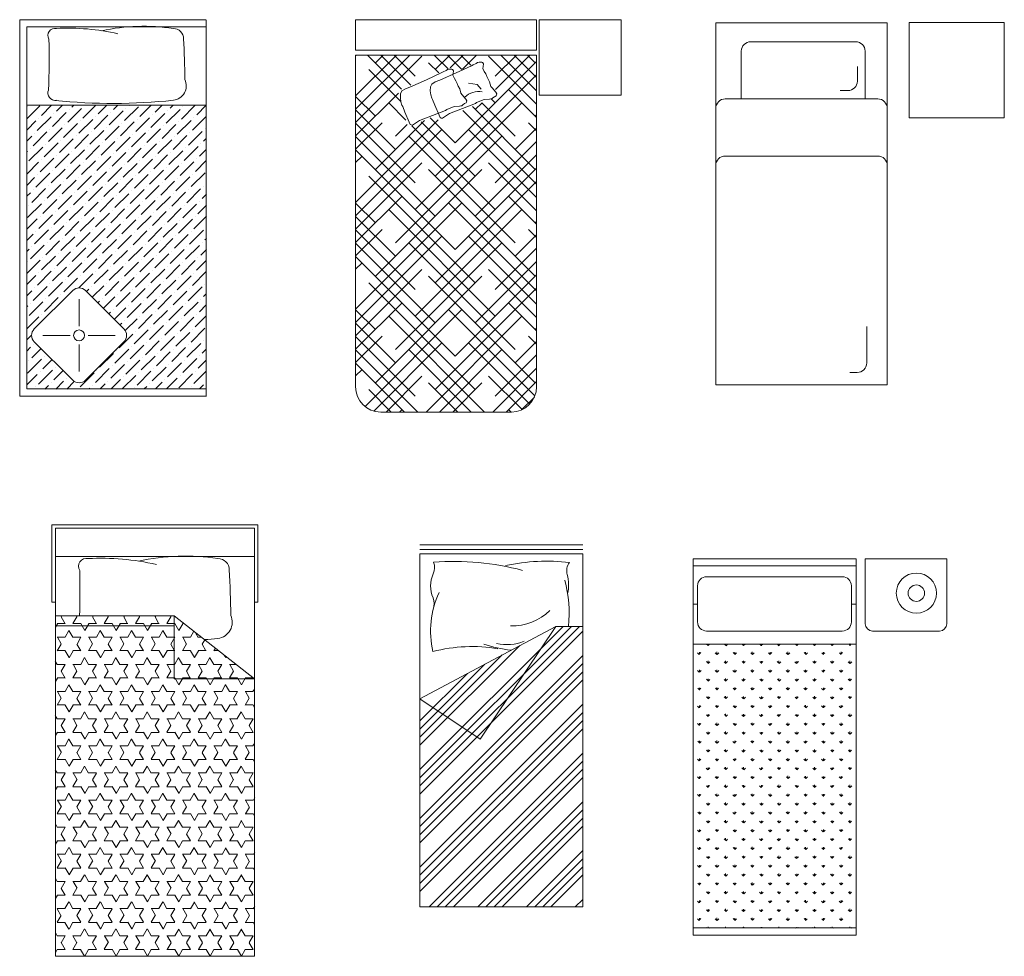
# Model space of a CAD drawing. Units: inches. Extents: x 1994 to 3075, y 3517 to 3950.
# Tile 20 of 58: x 1994.5453 to 1994.7595, y 3553.3484 to 3553.5521. Entities that reach past the tile are written whole.
import ezdxf

# ---------------------------------------------------------------- set-up
doc = ezdxf.new("R2010")
doc.units = ezdxf.units.IN
doc.layers.add('A-FURN-REFR', color=8, linetype='Continuous', lineweight=13)
doc.layers.add('A-FURN-REFR-PATT', color=8, linetype='Continuous', lineweight=13)

# ---------------------------------------------------------------- blocks, each defined once
blk = doc.blocks.new('*X5')
at = {"color": 0}
for p, q in [((-210.7580465308878, 409.7281539603075), (-199.9708546801334, 420.5153458110619)), ((-210.7580465308878, 412.379804389757), (-202.6225051095829, 420.5153458110619)), ((-210.7580465308878, 420.3347556781058), (-210.5774563979316, 420.5153458110619)), ((-210.7580465308878, 407.076503530858), (-197.547956993992, 420.2865930677537)), ((-201.617062875051, 413.7490972310152), (-208.3833114550977, 420.5153458110619)), ((-206.8287334970653, 418.9607678530292), (-205.2741555390325, 420.5153458110619)), ((-199.7682837993056, 414.5519685847194), (-205.7316610256482, 420.5153458110619)), ((-198.8737822087164, 416.3091174235798), (-203.0800105961986, 420.515345811062)), ((-192.3731674963244, 417.7634539995364), (-195.12505930785, 420.5153458110619)), ((-194.8963065645422, 417.6349426383045), (-192.0159033917846, 420.515345811062)), ((-189.6311998323742, 417.6731367650358), (-192.4734088784004, 420.515345811062)), ((-191.9188461243063, 417.9607526490907), (-189.3642529623351, 420.5153458110619)), ((-190.9188309203679, 403.0508652763318), (-174.7580465308877, 419.211649665812)), ((-187.8124935512899, 418.5060809134011), (-189.8217584489508, 420.5153458110619)), ((-189.4902654306947, 417.7376829132529), (-186.7126025328856, 420.5153458110619)), ((-174.7580465308877, 410.7549347518979), (-184.2897048467439, 420.2865930677541)), ((-182.9638796320193, 416.3091174235796), (-178.7576512445369, 420.5153458110619)), ((-182.9257945198644, 413.695552106285), (-176.1060008150873, 420.515345811062)), ((-174.7580465308877, 413.4065851813475), (-181.8668071606022, 420.5153458110619)), ((-174.7580465308877, 416.058235610797), (-179.2151567311527, 420.5153458110619)), ((-175.0089283436705, 418.9607678530292), (-176.5635063017031, 420.5153458110619)), ((-201.7778662022018, 411.2582501287165), (-208.1545587117899, 417.6349426383045)), ((-194.2219465720697, 416.9605826458322), (-196.2221317792669, 418.9607678530292)), ((-194.8963065645423, 396.421739202708), (-174.7580465308877, 416.5599992363624)), ((-174.7580465308877, 408.1032843224484), (-180.3122292025696, 413.6574669941301)), ((-210.7580465308878, 404.4248531014084), (-202.2434538897721, 412.9394457425241)), ((-206.8287334970651, 408.3541661352311), (-210.7580465308878, 412.2834791690537)), ((-182.9638796320191, 411.0058165646806), (-183.727333396784, 411.7692703294456)), ((-202.8512578528907, 401.7250400616072), (-210.7580465308877, 409.6318287396042)), ((-200.7622625975809, 407.590996094646), (-204.1770830676156, 411.0058165646806)), ((-198.8737822087168, 389.7926131290839), (-177.6605787731203, 411.0058165646803)), ((-174.7580465308877, 394.8450321752006), (-189.4137563576908, 409.5007420020037)), ((-175.0089283436705, 397.7475644174329), (-187.5182820373886, 410.256918111151)), ((-186.9413552761936, 409.6799913499556), (-185.5985917406192, 411.02275488553)), ((-178.9864039878448, 404.3766904910567), (-185.6228077170863, 411.0130942202982)), ((-210.7580465308878, 391.1666009541607), (-194.3064165629733, 407.6182309220751)), ((-206.8287334970653, 397.7475644174327), (-197.0508686209985, 407.5254292934994)), ((-190.9188309203678, 403.050865276332), (-195.8995790361304, 408.0316133920946)), ((-175.0089283436706, 408.3541661352309), (-174.7580465308877, 408.6050479480137)), ((-210.7580465308878, 401.7732026719589), (-205.5029082823405, 407.0283409205061)), ((-198.8737822087164, 395.0959139879834), (-210.7580465308878, 406.9801783101546)), ((-210.7580465308878, 388.5149505247111), (-193.5704813498175, 405.7025157057813)), ((-202.851257852891, 404.3766904910565), (-200.5182087880894, 406.7097395558581)), ((-182.9638796320191, 389.7926131290843), (-199.583278575489, 406.4120120725541)), ((-186.9413552761934, 396.4217392027081), (-197.7414288058097, 407.2218127323244)), ((-174.7580465308877, 392.1933817457511), (-188.2671804909182, 405.7025157057815)), ((-178.9864039878449, 401.7250400616069), (-174.7580465308877, 405.9533975185642)), ((-174.7580465308877, 405.4516338929988), (-176.3347535583952, 407.0283409205063)), ((-194.8963065645421, 388.4667879143594), (-210.7580465308878, 404.328527880705)), ((-202.8512578528911, 383.16348705546), (-181.6380544172947, 404.3766904910564)), ((-178.9864039878448, 383.1634870554603), (-200.1996074234412, 404.3766904910567)), ((-190.9188309203678, 381.8376618407356), (-210.7580465308878, 401.6768774512555)), ((-182.9638796320193, 395.0959139879831), (-174.7580465308877, 403.3017470891146)), ((-210.7580465308878, 399.1215522425094), (-209.4803839265148, 400.3992148468823)), ((-186.9413552761938, 388.4667879143591), (-174.7580465308877, 400.6500966596651)), ((-210.7580465308878, 385.8633000952616), (-197.5479569939918, 399.0733896321575)), ((-206.8287334970653, 376.5343609818363), (-185.6155300614688, 397.7475644174327)), ((-175.0089283436705, 376.5343609818365), (-196.2221317792669, 397.7475644174329)), ((-190.9188309203679, 381.8376618407354), (-174.7580465308877, 397.9984462302155)), ((-174.7580465308877, 389.5417313163016), (-184.2897048467439, 399.0733896321577)), ((-186.9413552761934, 375.2085357671117), (-208.1545587117898, 396.4217392027081)), ((-194.8963065645423, 375.2085357671115), (-174.7580465308877, 395.346795800766)), ((-210.7580465308878, 383.211649665812), (-201.5254326381662, 392.4442635585336)), ((-174.7580465308877, 386.890080886852), (-180.3122292025696, 392.4442635585338)), ((-210.7580465308878, 369.9533975185643), (-189.5930057056432, 391.1184383438088)), ((-206.8287334970651, 387.1409626996347), (-210.7580465308878, 391.0702757334573)), ((-182.9638796320191, 368.5794096934878), (-204.1770830676156, 389.7926131290843)), ((-198.8737822087166, 368.5794096934876), (-177.6605787731202, 389.792613129084)), ((-174.7580465308877, 373.6318287396042), (-192.2446561350925, 391.118438343809)), ((-202.8512578528907, 380.5118366260108), (-210.7580465308877, 388.4186253040078)), ((-175.0089283436706, 387.1409626996345), (-174.7580465308877, 387.3918445124174)), ((-210.7580465308878, 380.5599992363625), (-205.5029082823405, 385.8151374849098)), ((-198.8737822087164, 373.8827105523869), (-210.7580465308877, 385.7669748745582)), ((-210.7580465308878, 367.3017470891147), (-193.5704813498175, 384.4893122701849)), ((-174.7580465308877, 370.9801783101547), (-188.2671804909182, 384.4893122701852)), ((-178.986403987845, 380.5118366260106), (-174.7580465308878, 384.7401940829678)), ((-174.7580465308877, 384.2384304574025), (-176.3347535583952, 385.81513748491)), ((-194.8963065645421, 367.253584478763), (-210.7580465308878, 383.1153244451087)), ((-202.8512578528909, 361.9502836198638), (-181.6380544172945, 383.1634870554602)), ((-178.9864039878448, 361.9502836198639), (-200.1996074234412, 383.1634870554603)), ((-182.9638796320192, 373.8827105523869), (-174.7580465308877, 382.0885436535184)), ((-190.9188309203678, 360.6244584051392), (-210.7580465308877, 380.4636740156592)), ((-210.7580465308878, 377.9083488069129), (-209.480383926515, 379.1860114112858)), ((-186.9413552761936, 367.2535844787628), (-174.7580465308877, 379.4368932240687)), ((-210.7580465308878, 364.6500966596652), (-197.547956993992, 377.8601861965609)), ((-206.8287334970653, 355.3211575462399), (-185.6155300614688, 376.5343609818363)), ((-175.0089283436705, 355.32115754624), (-196.2221317792669, 376.5343609818365)), ((-190.9188309203679, 360.624458405139), (-174.7580465308877, 376.7852427946191)), ((-174.7580465308877, 368.3285278807051), (-184.2897048467439, 377.8601861965612)), ((-186.9413552761935, 353.9953323315153), (-208.1545587117899, 375.2085357671118)), ((-194.8963065645423, 353.9953323315151), (-174.7580465308878, 374.1335923651696)), ((-210.7580465308878, 361.9984462302156), (-201.5254326381662, 371.2310601229372)), ((-174.7580465308877, 365.6768774512556), (-180.3122292025696, 371.2310601229374)), ((-206.8287334970651, 365.9277592640383), (-210.7580465308877, 369.8570722978609)), ((-208.8846967480148, 350.6135438658409), (-189.5930057056432, 369.9052349082124)), ((-185.1130191851898, 349.5153458110621), (-204.1770830676156, 368.5794096934878)), ((-196.7246426555458, 349.5153458110621), (-177.6605787731202, 368.5794096934877)), ((-175.0826291794211, 352.7432079525412), (-192.2446561350925, 369.9052349082126)), ((-202.8512578528908, 359.2986331904144), (-210.7580465308877, 367.2054218684114)), ((-210.7580465308878, 359.3467958007661), (-205.5029082823405, 364.6019340493134)), ((-198.8737822087165, 352.6695071167905), (-210.7580465308878, 364.5537714389618)), ((-174.7580465308877, 363.025227021806), (-176.3347535583952, 364.6019340493135)), ((-175.0089283436707, 365.9277592640381), (-174.7580465308878, 366.1786410768209)), ((-207.1372587068342, 349.7093314775719), (-193.5704813498174, 363.2761088345887)), ((-176.0989374029306, 351.1078657466011), (-188.2671804909182, 363.2761088345887)), ((-178.986403987845, 359.2986331904143), (-174.7580465308878, 363.5269906473715)), ((-198.3712713324375, 349.5153458110621), (-210.7580465308878, 361.9021210095123)), ((-187.7646696146393, 349.5153458110621), (-200.1996074234413, 361.950283619864)), ((-194.0729922260963, 349.5153458110621), (-181.6380544172946, 361.9502836198638)), ((-182.9638796320193, 352.6695071167903), (-174.7580465308878, 360.8753402179218)), ((-201.0229217618871, 349.5153458110621), (-210.7580465308878, 359.2504705800627)), ((-210.7580465308878, 356.6951453713165), (-209.4803839265148, 357.9728079756894)), ((-204.6795939438944, 349.5153458110621), (-197.5479569939918, 356.6469827609647)), ((-177.6324032389686, 349.9896811531895), (-184.2897048467439, 356.6469827609648)), ((-183.4663905082981, 349.5153458110621), (-174.7580465308878, 358.2236897884723)), ((-190.4163200440889, 349.5153458110621), (-196.2221317792669, 355.3211575462401)), ((-191.4213417966468, 349.5153458110621), (-185.6155300614689, 355.3211575462399)), ((-180.8147400788485, 349.5153458110621), (-174.7580465308878, 355.5720393590228)), ((-203.6745721913366, 349.5153458110621), (-208.1545587117899, 353.9953323315153)), ((-177.7359644727731, 349.942470987688), (-175.1851717075138, 352.4932637529473)), ((-202.0279435144449, 349.5153458110621), (-201.5254326381662, 350.0178566873408)), ((-179.8097183262906, 349.5153458110621), (-180.3122292025696, 350.017856687341))]:
    blk.add_line(p, q, dxfattribs=at)

msp = doc.modelspace()

# ---------------------------------------------------------------- hatches: boundary and pattern name
at = {"layer": 'A-FURN-REFR-PATT'}
h = msp.add_hatch(dxfattribs=at)
h.set_pattern_fill('ANSI36', color=256, scale=0.0005368647100931, style=0)
h.set_pattern_definition([(45, (1992.896359554233, 3553.126432773951), (0.0009039717373123, 0.0033145630368119), [0.0042613636363636, -0.0008522727272727, 0, -0.0008522727272727])])
h.paths.add_polyline_path([(1994.546861451254, 3553.471827593295), (1994.585872349944, 3553.471827593295), (1994.585872349944, 3553.533572260688), (1994.546861451254, 3553.533572260688)])
h.paths.add_polyline_path([(1994.559597014725, 3553.493218537151), (1994.567948669621, 3553.484866882255, -0.4142135623730951), (1994.567948669621, 3553.48208299729), (1994.559597014725, 3553.473731342394, -0.4142135623730951), (1994.55681312976, 3553.473731342394), (1994.548461474864, 3553.48208299729, -0.4142135623730951), (1994.548461474864, 3553.484866882255), (1994.55681312976, 3553.493218537151, -0.4142135623730949)], flags=16)
h = msp.add_hatch(dxfattribs=at)
h.set_pattern_fill('STARS', color=256, scale=0.0005368647100931, style=0)
h.set_pattern_definition([(0, (1993.050049029089, 3553.090100364233), (0, 0.0029523586256263), [0.0017045454545455, -0.0017045454545455]), (60, (1993.050049029089, 3553.090100364233), (-0.0025568175708745, 0.0014761793128132), [0.0017045454545455, -0.0017045454545455]), (119.9999999999999, (1993.050901301817, 3553.091576543546), (-0.0025568175708745, -0.0014761793128132), [0.0017045454545455, -0.0017045454545455])])
h.paths.add_polyline_path([(1994.553043561207, 3553.348413258822), (1994.596372491915, 3553.348413258822), (1994.596372491915, 3553.408773288821), (1994.578910061208, 3553.408773288821), (1994.578910061208, 3553.420293288821), (1994.553043561207, 3553.420293288821)])
h.paths.add_polyline_path([(1994.596372491915, 3553.408773288821), (1994.578910061208, 3553.422453288821), (1994.578910061208, 3553.408773288821)])
h.paths.add_polyline_path([(1994.578910061208, 3553.420293288821), (1994.578910061208, 3553.422453288821), (1994.553043561207, 3553.422453288821), (1994.553043561207, 3553.420293288821)])
h = msp.add_hatch(dxfattribs=at)
h.set_pattern_fill('ANSI34', color=256, scale=0.0003937007874016, style=0)
h.set_pattern_definition([(45, (1993.050049029089, 3553.090100364233), (-0.0053033008588991, 0.0053033008588991), []), (45, (1993.051816796806, 3553.090100364233), (-0.0053033008588991, 0.0053033008588991), []), (45, (1993.053584564523, 3553.090100364233), (-0.0053033008588991, 0.0053033008588991), []), (45, (1993.055352336176, 3553.090100364233), (-0.0053033008588991, 0.0053033008588991), [])])
h.paths.add_polyline_path([(1994.632359589973, 3553.404436820766), (1994.645437540004, 3553.395663695953), (1994.661887149027, 3553.420184852262)], flags=17)
h.paths.add_polyline_path([(1994.645437540004, 3553.395663695953), (1994.632359589973, 3553.404436820766), (1994.632359589973, 3553.359161230215), (1994.667792660839, 3553.359161230215), (1994.667792660839, 3553.420184852262), (1994.661887149027, 3553.420184852262)])
h = msp.add_hatch(dxfattribs=at)
h.set_pattern_fill('GRASS', color=256, scale=0.0001073729420186, style=0)
h.set_pattern_definition([(90, (1993.050049029089, 3553.090100364233), (-0.0019284717251253, 0.0019284717251253), [0.0005113636363636, -0.0033455798138869]), (45, (1993.050049029089, 3553.090100364233), (-0.0019284730395997, 0.0019284730395997), [0.0005113636363636, -0.0022159090909091]), (135, (1993.050049029089, 3553.090100364233), (-0.0019284730395997, -0.0019284730395997), [0.0005113636363636, -0.0022159090909091])])
h.paths.add_polyline_path([(1994.69181488028, 3553.354574789245), (1994.727247951146, 3553.354574789245), (1994.727247951146, 3553.416319456637), (1994.69181488028, 3553.416319456637)])

# ---------------------------------------------------------------- linework, layer by layer
at = {"layer": 'A-FURN-REFR'}
for p, q in [((1994.545286648104, 3553.470252790145), (1994.545286648104, 3553.552142553924)), ((1994.585872349944, 3553.552142553924), (1994.545286648104, 3553.552142553924)), ((1994.546861451254, 3553.471827593295), (1994.546861451254, 3553.550567750775)), ((1994.585872349944, 3553.550567750775), (1994.546861451254, 3553.550567750775)), ((1994.585872349944, 3553.470157443203), (1994.585872349944, 3553.552047206982)), ((1994.696695721813, 3553.551494491247), (1994.733993691145, 3553.551494491247)), ((1994.696695721813, 3553.472754333767), (1994.696695721813, 3553.551494491247)), ((1994.733993691145, 3553.472754333767), (1994.733993691145, 3553.551494491247)), ((1994.696695721813, 3553.536989725396), (1994.696695721813, 3553.54942238184)), ((1994.727127375017, 3553.547351280916), (1994.704334171536, 3553.547351280916)), ((1994.702262062128, 3553.534918624472), (1994.702262062128, 3553.545279171509)), ((1994.729199484424, 3553.534918624472), (1994.729199484424, 3553.545279171509)), ((1994.727496280641, 3553.541967400785), (1994.727496280641, 3553.538785783707)), ((1994.642927317379, 3553.538302041658), (1994.64481344291, 3553.538032798672)), ((1994.64481344291, 3553.538032798672), (1994.645655457301, 3553.537023135932)), ((1994.723796114248, 3553.536713674299), (1994.725424171233, 3553.536713674299)), ((1994.585872349944, 3553.533572260688), (1994.546861451254, 3553.533572260688)), ((1994.69876783122, 3553.534917615988), (1994.731921581738, 3553.534917615988)), ((1994.69876783122, 3553.522484959544), (1994.731921581738, 3553.522484959544)), ((1994.55681312976, 3553.493218537151), (1994.548461474864, 3553.484866882255)), ((1994.567948669621, 3553.484866882255), (1994.559597014725, 3553.493218537151)), ((1994.558205072243, 3553.49134895552), (1994.558205072243, 3553.485443443709)), ((1994.729529637314, 3553.485432178256), (1994.729529637314, 3553.477467660849)), ((1994.548461474864, 3553.48208299729), (1994.55681312976, 3553.473731342394)), ((1994.550331056495, 3553.483474939773), (1994.556236568305, 3553.483474939773)), ((1994.559597014725, 3553.473731342394), (1994.567948669621, 3553.48208299729)), ((1994.56017357618, 3553.483474939773), (1994.566079087991, 3553.483474939773)), ((1994.558205072243, 3553.481506435836), (1994.558205072243, 3553.475600924024)), ((1994.725829470921, 3553.475395551441), (1994.727457527907, 3553.475395551441)), ((1994.546861451254, 3553.471827593295), (1994.585872349944, 3553.471827593295)), ((1994.696695721813, 3553.472754333767), (1994.733993691145, 3553.472754333767)), ((1994.545286648104, 3553.470252790145), (1994.585872349944, 3553.470252790145)), ((1994.552293561208, 3553.425413288821), (1994.552293561208, 3553.442288288821)), ((1994.552293561208, 3553.442288288821), (1994.597122491915, 3553.442288288821)), ((1994.553043561207, 3553.441538288821), (1994.596372491915, 3553.441538288821)), ((1994.553043561207, 3553.441538288821), (1994.553043561207, 3553.425413288821)), ((1994.596372491915, 3553.441538288821), (1994.596372491915, 3553.348413258822)), ((1994.597122491915, 3553.425447900457), (1994.597122491915, 3553.442288288821)), ((1994.667792660839, 3553.437901387695), (1994.632359589973, 3553.437901387695)), ((1994.632359589973, 3553.436917135726), (1994.667792660839, 3553.436917135726)), ((1994.553043561207, 3553.348413258822), (1994.553043561207, 3553.43541328882)), ((1994.553043561207, 3553.43541328882), (1994.596372491915, 3553.43541328882)), ((1994.632359589973, 3553.435932883758), (1994.667792660839, 3553.435932883758)), ((1994.632359589973, 3553.359161230215), (1994.632359589973, 3553.435932883758)), ((1994.667792660839, 3553.435932883758), (1994.667792660839, 3553.359161230215)), ((1994.69181488028, 3553.352999986095), (1994.69181488028, 3553.434889749875)), ((1994.727247951146, 3553.434889749875), (1994.69181488028, 3553.434889749875)), ((1994.727247951146, 3553.352999986095), (1994.727247951146, 3553.434889749875)), ((1994.746951834969, 3553.434889749875), (1994.729235299536, 3553.434889749875)), ((1994.729235299536, 3553.434889749875), (1994.729235299536, 3553.420734361488)), ((1994.746951834969, 3553.420734361488), (1994.746951834969, 3553.434889749875)), ((1994.727247951146, 3553.433314946725), (1994.69181488028, 3553.433314946725)), ((1994.724225196212, 3553.430983905812), (1994.694697637157, 3553.430983905812)), ((1994.69272913322, 3553.429015401875), (1994.69272913322, 3553.421141386126)), ((1994.726193700149, 3553.421141386126), (1994.726193700149, 3553.429015401875)), ((1994.553043561207, 3553.425413288821), (1994.552293561208, 3553.425413288821)), ((1994.597122491915, 3553.425447900457), (1994.596372491915, 3553.425447900457)), ((1994.69181488028, 3553.425022458472), (1994.69272913322, 3553.425022458472)), ((1994.726193700149, 3553.425022458472), (1994.727247951146, 3553.425022458472)), ((1994.553044761208, 3553.422453288821), (1994.578910061208, 3553.422453288821)), ((1994.578910061208, 3553.422453288821), (1994.578910061208, 3553.408773288821)), ((1994.596372491915, 3553.408773288821), (1994.578910061208, 3553.422453288821)), ((1994.578910061208, 3553.420293288821), (1994.553044761208, 3553.420293288821)), ((1994.632359589973, 3553.404436820766), (1994.661887149027, 3553.420184852262)), ((1994.645437540004, 3553.395663695953), (1994.661887149027, 3553.420184852262)), ((1994.661887149027, 3553.420184852262), (1994.667792660839, 3553.420184852262)), ((1994.694697637157, 3553.41917288219), (1994.724225196212, 3553.41917288219)), ((1994.730810102685, 3553.419159558337), (1994.745377031819, 3553.419159558337)), ((1994.727247951146, 3553.416319456637), (1994.69181488028, 3553.416319456637)), ((1994.578910061208, 3553.408773288821), (1994.596372491915, 3553.408773288821)), ((1994.632359589973, 3553.404436820766), (1994.645437540004, 3553.395663695953)), ((1994.667792660839, 3553.359161230215), (1994.632359589973, 3553.359161230215)), ((1994.69181488028, 3553.354574789245), (1994.727247951146, 3553.354574789245)), ((1994.69181488028, 3553.352999986095), (1994.727247951146, 3553.352999986095)), ((1994.553043561207, 3553.348413258822), (1994.596372491915, 3553.348413258822))]:
    msp.add_line(p, q, dxfattribs=at)
for points in [[(1994.657722327232, 3553.552107953363), (1994.618352248491, 3553.552107953363), (1994.618352248491, 3553.545546273574), (1994.657722327232, 3553.545546273574)], [(1994.676142643871, 3553.535703753888), (1994.676142643871, 3553.552107953363), (1994.658273068453, 3553.552107953363), (1994.658273068453, 3553.535703753888)], [(1994.759466637006, 3553.551512974404), (1994.759466637006, 3553.53079188033), (1994.738745542932, 3553.53079188033), (1994.738745542932, 3553.551512974404)], [(1994.647963488226, 3553.534943268839), (1994.648220532195, 3553.535135903115), (1994.648541830034, 3553.535392748817), (1994.64892739124, 3553.535585383093), (1994.649055917973, 3553.536034869217), (1994.64886313737, 3553.53635593249), (1994.648027751593, 3553.537319110017), (1994.647770707624, 3553.537640167145), (1994.647513663655, 3553.538603350818), (1994.647192356319, 3553.539181253647), (1994.646935321847, 3553.539759162621), (1994.646678277877, 3553.540337071596), (1994.646356970542, 3553.540850769146), (1994.646035672703, 3553.541557100972), (1994.64609993607, 3553.541942369525), (1994.64616418994, 3553.5425202785), (1994.646046973635, 3553.542743736964), (1994.645932330904, 3553.542827463205), (1994.645778628734, 3553.542905547052), (1994.645521584765, 3553.542905547052), (1994.645200286926, 3553.542905547052), (1994.64487897959, 3553.542841335627), (1994.644557681752, 3553.542584489925), (1994.643915076577, 3553.542327644223), (1994.643593769241, 3553.542135003801), (1994.640252226133, 3553.540593917298), (1994.636653639055, 3553.538988619371), (1994.635689726545, 3553.538603350818), (1994.634918604134, 3553.538153864694), (1994.634661560165, 3553.537511744294), (1994.634597296799, 3553.536676989617), (1994.634725823532, 3553.535778023515), (1994.634918604134, 3553.53507169169), (1994.635111384737, 3553.534750628415), (1994.635561209309, 3553.533530605187), (1994.636525112322, 3553.531347398285), (1994.636718576679, 3553.530858741163), (1994.636937311438, 3553.530749458197), (1994.63723235123, 3553.530717699756), (1994.638770218799, 3553.531750257252), (1994.644429155019, 3553.533915873739), (1994.644686198988, 3553.534108508016), (1994.646317703734, 3553.534748970875), (1994.647476427559, 3553.534877109005), (1994.647770707624, 3553.534943268839)], [(1994.641458045061, 3553.533433043404), (1994.64171508903, 3553.53362567768), (1994.642036386869, 3553.533882523381), (1994.642421948075, 3553.534075157657), (1994.642550474807, 3553.534524643782), (1994.642357694205, 3553.534845707055), (1994.641522308427, 3553.535808884582), (1994.641265264459, 3553.536129941709), (1994.641008220489, 3553.537093125382), (1994.640686913154, 3553.537671028212), (1994.640429878682, 3553.538248937186), (1994.640172834712, 3553.538826846161), (1994.639851527377, 3553.539340543711), (1994.639530229538, 3553.540046875536), (1994.639594492904, 3553.540432144089), (1994.639658746774, 3553.541010053064), (1994.63954153047, 3553.541233511528), (1994.639426887739, 3553.541317237769), (1994.639273185569, 3553.541395321616), (1994.6390161416, 3553.541395321616), (1994.63869484376, 3553.541395321616), (1994.638373536425, 3553.541331110191), (1994.638052238586, 3553.541074264489), (1994.637409633412, 3553.540817418788), (1994.637088326076, 3553.540624778365), (1994.633746782968, 3553.539083691863), (1994.63014819589, 3553.537478393935), (1994.62918428338, 3553.537093125382), (1994.628413160969, 3553.536643639259), (1994.628156117, 3553.536001518858), (1994.628091853634, 3553.535166764182), (1994.628220380366, 3553.53426779808), (1994.628413160969, 3553.533561466255), (1994.628605941572, 3553.533240402981), (1994.629055766144, 3553.532020379752), (1994.630019669157, 3553.529837172849), (1994.630213133514, 3553.529348515727), (1994.630431868273, 3553.529239232761), (1994.630726908065, 3553.52920747432), (1994.632264775634, 3553.530240031817), (1994.637923711853, 3553.532405648303), (1994.638180755822, 3553.53259828258), (1994.639812260568, 3553.533238745439), (1994.640970984393, 3553.533366883569), (1994.641265264459, 3553.533433043404)]]:
    msp.add_lwpolyline(points, close=True, dxfattribs=at)
msp.add_lwpolyline([(1994.657722327232, 3553.472274182585), (1994.657722327232, 3553.544452660275), (1994.618352248491, 3553.544452660275), (1994.618352248491, 3553.472274182585, 0.4142135623730951), (1994.623820314983, 3553.466806116093), (1994.65225426074, 3553.466806116093, 0.4142135623730951)], format="xyb", close=True, dxfattribs=at)
for centre, radius in [((1994.558205072243, 3553.483474939773), 0.0011811023622047), ((1994.740341013666, 3553.427406071231), 0.0043699566549229), ((1994.740341013666, 3553.427406071231), 0.0017877096733892)]:
    msp.add_circle(centre, radius, dxfattribs=at)
for centre, radius, start, end in [((1994.552975734361, 3553.548710572547), 0.0015495648594936, 78.72778623498706, 211.6094986857782), ((1994.552975734361, 3553.548710572547), 0.0015495648594936, 78.72778623498706, 211.6094986857782), ((1994.555846077112, 3553.502026513773), 0.048272057721766, 77.05638185161688, 93.04883220562752), ((1994.555846077112, 3553.502026513773), 0.048272057721766, 77.05638185161688, 93.04883220562752), ((1994.572258072299, 3553.507218279324), 0.0434930463328828, 81.47022635647696, 102.1032641982298), ((1994.572258072299, 3553.507218279324), 0.0434930463328828, 81.47022635647696, 102.1032641982298), ((1994.578709105823, 3553.54800042039), 0.002229825242405, 0, 90), ((1994.578709105823, 3553.54800042039), 0.002229825242405, 0, 90), ((1994.392063358424, 3553.543987585989), 0.159640614517258, 357.4333292641344, 1.403751564921032), ((1994.392063358424, 3553.543987585989), 0.159640614517258, 357.4333292641344, 1.403751564921032), ((1994.315715921451, 3553.534870785229), 0.2655477963543014, 0.9125644663952034, 2.834064295864955), ((1994.315715921451, 3553.534870785229), 0.2655477963543014, 0.9125644663952034, 2.834064295864955), ((1994.704334171536, 3553.545279171509), 0.0020721094073767, 90, 180), ((1994.727127375017, 3553.545279171509), 0.0020721094073767, 0, 90), ((1994.578318741922, 3553.537781001943), 0.0031961751250146, 277.015318444972, 24.37436785420747), ((1994.578318741922, 3553.537781001943), 0.0031961751250146, 277.015318444972, 24.37436785420747), ((1994.725424171233, 3553.538785783707), 0.0020721094073767, 270, 0), ((1994.725424171233, 3553.538785783707), 0.0020721094073767, 270, 0), ((1994.553009671983, 3553.536189261227), 0.0016032273792557, 156.1084115545774, 279.6575795622506), ((1994.553009671983, 3553.536189261227), 0.0016032273792557, 156.1084115545774, 279.6575795622506), ((1994.645151119757, 3553.53210716321), 0.0043972037208896, 80.65587160230488, 133.423915418803), ((1994.565750140694, 3553.658166503273), 0.1242354698394082, 264.1139139330622, 275.9873971424126), ((1994.565750140694, 3553.658166503273), 0.1242354698394082, 264.1139139330622, 275.9873971424126), ((1994.69876783122, 3553.532845506581), 0.0020721094073767, 90, 180), ((1994.731921581738, 3553.532845506581), 0.0020721094073767, 0, 90), ((1994.69876783122, 3553.520412850136), 0.0020721094073767, 90, 180), ((1994.731921581738, 3553.520412850136), 0.0020721094073767, 0, 90), ((1994.558205072243, 3553.491826594668), 0.0019685039370078, 45, 135), ((1994.549853417347, 3553.483474939773), 0.0019685039370079, 135, 225), ((1994.566556727139, 3553.483474939773), 0.0019685039370079, 315, 45), ((1994.727457527907, 3553.477467660849), 0.0020721094073767, 270, 0), ((1994.727457527907, 3553.477467660849), 0.0020721094073767, 270, 0), ((1994.558205072243, 3553.475123284876), 0.0019685039370079, 225, 315), ((1994.559817138509, 3553.433238175312), 0.0017217387327707, 78.72778623498706, 211.6094986857782), ((1994.559817138509, 3553.433238175312), 0.0017217387327707, 78.72778623498706, 211.6094986857782), ((1994.563006408232, 3553.381366998897), 0.0536356196908511, 77.05638185161688, 93.04883220562752), ((1994.563006408232, 3553.381366998897), 0.0536356196908511, 77.05638185161688, 93.04883220562752), ((1994.58124195844, 3553.387135627286), 0.0483256070365364, 81.47022635647696, 102.1032641982298), ((1994.58124195844, 3553.387135627286), 0.0483256070365364, 81.47022635647696, 102.1032641982298), ((1994.588409773467, 3553.43244911736), 0.0024775836026722, 0, 90), ((1994.588409773467, 3553.43244911736), 0.0024775836026722, 0, 90), ((1994.296195124164, 3553.417860633847), 0.2950531070603349, 0.9125644663952034, 2.834064295864955), ((1994.296195124164, 3553.417860633847), 0.2950531070603349, 0.9125644663952034, 2.834064295864955), ((1994.632333975953, 3553.432936270738), 0.0032028341489732, 335.7877323280015, 21.71237864400314), ((1994.63992190676, 3553.377803303817), 0.0565064023996118, 74.89247536308716, 94.681970907379), ((1994.659901603531, 3553.392894067574), 0.0414680575843914, 83.14136388124066, 102.4247502365447), ((1994.667379773442, 3553.432255481189), 0.0031075126812102, 144.3787648229011, 195.1987658355305), ((1994.381025609691, 3553.427990412471), 0.1773784605747312, 358.2111392619709, 1.403751564921032), ((1994.381025609691, 3553.427990412471), 0.1773784605747312, 358.2111392619709, 1.403751564921032), ((1994.641253015378, 3553.42892559989), 0.0065764677133891, 155.7877323280015, 202.8808293159797), ((1994.634945753122, 3553.422873271051), 0.0298558147000044, 354.833703975234, 14.25995084780135), ((1994.65608535557, 3553.429187117011), 0.0085962787467616, 347.311957921453, 15.19876583553051), ((1994.694697637157, 3553.429015401875), 0.0019685039370078, 90, 180), ((1994.724225196212, 3553.429015401875), 0.0019685039370078, 0, 90), ((1994.654520157182, 3553.419162370253), 0.0198519972069101, 155.1179531461462, 192.9861889591517), ((1994.63211664709, 3553.425069848737), 0.0033401870886801, 339.0160855821216, 22.88082931597971), ((1994.587976035799, 3553.421094207974), 0.0035513056944607, 277.015318444972, 24.37436785420747), ((1994.587976035799, 3553.421094207974), 0.0035513056944607, 277.015318444972, 24.37436785420747), ((1994.652514080446, 3553.43175405124), 0.0114567055564695, 267.8294752673963, 315.0098308273483), ((1994.694697637157, 3553.421141386126), 0.0019685039370081, 180, 270), ((1994.724225196212, 3553.421141386126), 0.0019685039370081, 270, 0), ((1994.730810102685, 3553.420734361488), 0.0015748031496063, 180, 270), ((1994.745377031819, 3553.420734361488), 0.0015748031496063, 270, 0), ((1994.574010923324, 3553.554855876118), 0.1380394109326758, 274.7720352878431, 275.9873971424126), ((1994.574010923324, 3553.554855876118), 0.1380394109326758, 274.7720352878431, 275.9873971424126), ((1994.643668402019, 3553.382091775515), 0.0336972432594088, 80.32657587842615, 104.5973118255227), ((1994.654508551833, 3553.439542997824), 0.0246390736856652, 250.3559327023518, 264.6012463476583), ((1994.651250357437, 3553.42619345329), 0.009989213432703, 257.148031947205, 292.3825063085086)]:
    msp.add_arc(centre, radius, start, end, dxfattribs=at)

# ---------------------------------------------------------------- block references
at = {"layer": 'A-FURN-REFR', "xscale": 0.0010936132983375, "yscale": 0.0010936132983375, "zscale": 0.0010936132983375}
msp.add_blockref('*X5', (1994.848840050909, 3553.084571485941), dxfattribs=at)

doc.saveas('drawing.dxf')
